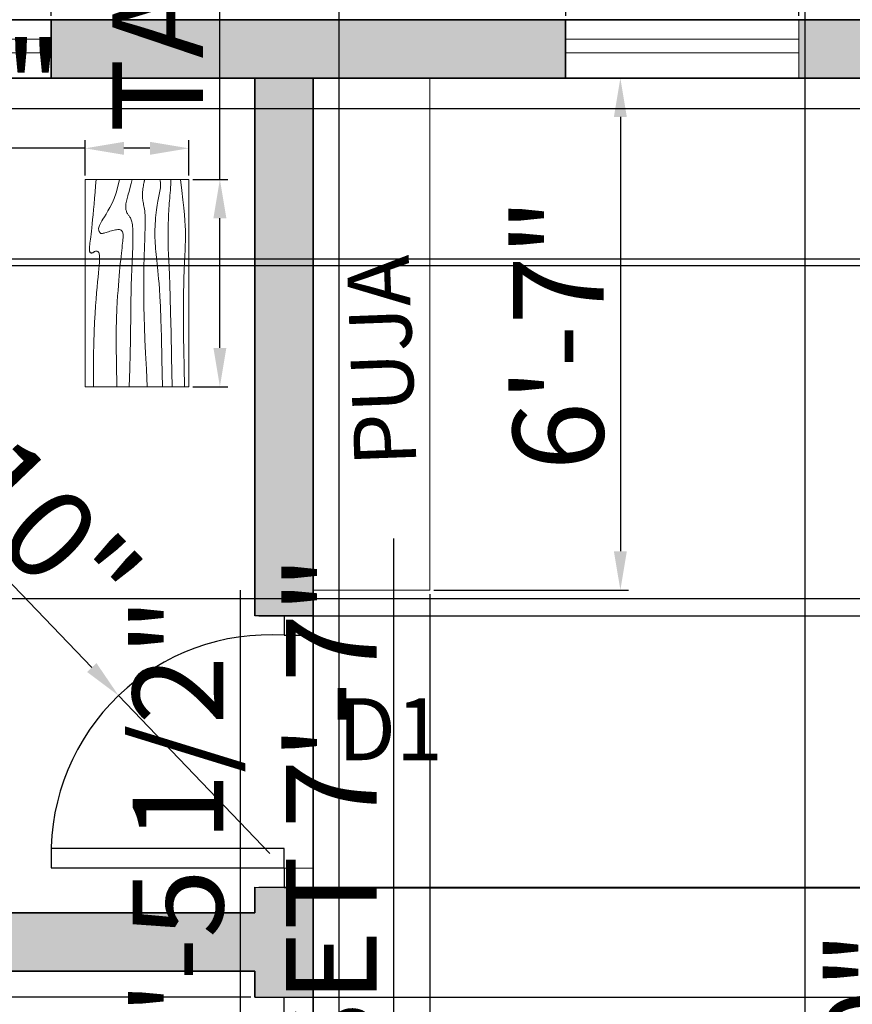
# Model space of a CAD drawing. Units: inches. Extents: x 2961 to 3748, y 1432 to 1961.
# Tile 6 of 9: x 3219 to 3348, y 1713 to 1865. Entities that reach past the tile are written whole.
import ezdxf
from ezdxf.enums import TextEntityAlignment as Align

# ---------------------------------------------------------------- set-up
doc = ezdxf.new("R2010")
doc.units = ezdxf.units.IN
for name, color, linetype, lineweight in [('A-ANNO-DIMS', 2, 'Continuous', 18), ('A-ANNO-TEXT', 7, 'Continuous', 18), ('A-AREA-IDEN', 7, 'Continuous', 18), ('A-DOOR', 3, 'Continuous', 25), ('A-FURN', 8, 'Continuous', 18), ('A-FURN-FIXD', 9, 'Continuous', 20), ('A-GLAZ', 4, 'Continuous', 18), ('A-WALL', 7, 'Continuous', 35), ('A-WALL-PATT', 252, 'Continuous', 13)]:
    doc.layers.add(name, color=color, linetype=linetype, lineweight=lineweight)
doc.styles.get("Standard").update_dxf_attribs({"font": 'arial.ttf'})
doc.dimstyles.new('ISO-25', dxfattribs={"dimtxt": 14, "dimasz": 6, "dimexe": 1.25, "dimexo": 0.625, "dimtad": 1, "dimlunit": 3, "dimtxsty": 'Standard', "dimcen": 2.5, "dimadec": 0, "dimazin": 0, "dimtfac": 1, "dimtmove": 0, "dimatfit": 3, "dimfxl": 1, "dimarcsym": 0})

# ---------------------------------------------------------------- blocks, each defined once
blk = doc.blocks.new('Table - Rectangular Woodgrain 60 x 30 in.')
for p, q in [((0, 0), (0, -30)), ((60, 0), (0, 0)), ((60, -30), (60, 0)), ((0, -30), (60, -30))]:
    blk.add_line(p, q)
for points in [[(0, -2.4), (4.8155, -2.418), (9.0302, -2.4688), (12.709, -2.5477), (15.9167, -2.65), (18.7181, -2.7711), (21.1781, -2.9063), (23.3616, -3.0508), (25.3333, -3.2), (27.1477, -3.3495), (28.8172, -3.4958), (30.3437, -3.636), (31.7291, -3.7667), (32.9756, -3.8849), (34.0849, -3.9875), (35.059, -4.0714), (35.9, -4.1334), (36.6114, -4.1711), (37.2041, -4.1854), (37.6906, -4.1779), (38.0833, -4.15), (38.3948, -4.1034), (38.6375, -4.0396), (38.8239, -3.9602), (38.9666, -3.8667), (39.0764, -3.7608), (39.1573, -3.6448), (39.2116, -3.521), (39.2416, -3.3917), (39.2498, -3.2593), (39.2385, -3.1261), (39.21, -2.9944), (39.1666, -2.8667), (39.111, -2.7447), (39.0468, -2.6281), (38.978, -2.5163), (38.9083, -2.4083), (38.8418, -2.3035), (38.7823, -2.201), (38.7337, -2.1001), (38.7, -2), (38.6844, -1.9003), (38.6875, -1.8021), (38.7094, -1.707), (38.75, -1.6167), (38.8094, -1.5326), (38.8875, -1.4563), (38.9844, -1.3893), (39.1, -1.3333), (39.2351, -1.2896), (39.3937, -1.2583), (39.5804, -1.2396), (39.8, -1.2333), (40.057, -1.2396), (40.3562, -1.2583), (40.7023, -1.2896), (41.1, -1.3333), (41.5547, -1.3895), (42.0755, -1.4573), (42.6721, -1.5361), (43.3542, -1.625), (44.1316, -1.7233), (45.014, -1.8302), (46.0114, -1.9449), (47.1333, -2.0667), (48.3862, -2.1947), (49.7625, -2.3281), (51.2513, -2.4663), (52.8416, -2.6083), (54.5226, -2.7535), (56.2833, -2.9011), (58.1127, -3.0501), (60, -3.2)], [(0, -9.2), (6.5759, -9.0858), (11.9385, -9.0365), (16.2527, -9.0418), (19.6833, -9.0917), (22.3952, -9.1759), (24.5531, -9.2844), (26.322, -9.4069), (27.8666, -9.5333), (29.3241, -9.6553), (30.7203, -9.7719), (32.0532, -9.8837), (33.3208, -9.9917), (34.5213, -10.0965), (35.6526, -10.199), (36.7128, -10.2999), (37.7, -10.4), (38.6129, -10.4996), (39.4531, -10.5969), (40.223, -10.6895), (40.925, -10.775), (41.5613, -10.8512), (42.1344, -10.9156), (42.6465, -10.966), (43.1, -11), (43.4976, -11.0158), (43.8437, -11.0136), (44.143, -10.9942), (44.4, -10.9583), (44.6195, -10.9069), (44.8062, -10.8406), (44.9648, -10.7603), (45.1, -10.6667), (45.2155, -10.5598), (45.3114, -10.4365), (45.3871, -10.2929), (45.4416, -10.125), (45.4743, -9.929), (45.4844, -9.7011), (45.4709, -9.4371), (45.4333, -9.1333), (45.3716, -8.7883), (45.2896, -8.4104), (45.1919, -8.0107), (45.0833, -7.6), (44.9685, -7.1893), (44.8521, -6.7896), (44.7388, -6.4117), (44.6333, -6.0667), (44.54, -5.7628), (44.4614, -5.4979), (44.4001, -5.2675), (44.3583, -5.0667), (44.3384, -4.8909), (44.3427, -4.7354), (44.3736, -4.5956), (44.4333, -4.4667), (44.5236, -4.3453), (44.6427, -4.2333), (44.7884, -4.1339), (44.9583, -4.05), (45.1501, -3.9849), (45.3614, -3.9417), (45.59, -3.9234), (45.8333, -3.9333), (46.0915, -3.9749), (46.3734, -4.0531), (46.6906, -4.1736), (47.0542, -4.3417), (47.4756, -4.5629), (47.9661, -4.8427), (48.5372, -5.1866), (49.2, -5.6), (49.9676, -6.0844), (50.8594, -6.625), (51.8965, -7.2031), (53.1, -7.8), (54.491, -8.3969), (56.0906, -8.975), (57.9199, -9.5156), (60, -10)], [(0, -12.8), (5.1847, -12.9322), (9.6213, -13.0323), (13.3963, -13.1059), (16.5958, -13.1583), (19.3063, -13.1952), (21.614, -13.2219), (23.6054, -13.2439), (25.3666, -13.2667), (26.9728, -13.2947), (28.4531, -13.3281), (29.8256, -13.3663), (31.1083, -13.4083), (32.3191, -13.4535), (33.476, -13.501), (34.597, -13.5501), (35.7, -13.6), (36.7984, -13.6497), (37.8875, -13.6979), (38.9578, -13.743), (40, -13.7833), (41.0047, -13.8174), (41.9625, -13.8438), (42.864, -13.8607), (43.7, -13.8667), (44.4631, -13.8604), (45.1552, -13.8417), (45.7801, -13.8104), (46.3416, -13.7667), (46.8439, -13.7104), (47.2906, -13.6417), (47.6858, -13.5604), (48.0333, -13.4667), (48.3375, -13.3608), (48.6042, -13.2448), (48.8396, -13.121), (49.05, -12.9917), (49.2417, -12.8593), (49.4208, -12.7261), (49.5937, -12.5944), (49.7667, -12.4667), (49.9452, -12.3451), (50.1323, -12.2313), (50.3303, -12.1268), (50.5416, -12.0333), (50.7686, -11.9524), (51.0135, -11.8854), (51.2788, -11.8341), (51.5666, -11.8), (51.8785, -11.7843), (52.2116, -11.7865), (52.562, -11.8059), (52.926, -11.8417), (53.2998, -11.8931), (53.6795, -11.9594), (54.0614, -12.0397), (54.4416, -12.1333), (54.8223, -12.2401), (55.2293, -12.3625), (55.6942, -12.5037), (56.2489, -12.6667), (56.9251, -12.8547), (57.7545, -13.0708), (58.7689, -13.3182), (60, -13.6)], [(0, -18), (5.124, -17.7273), (9.6609, -17.5057), (13.6705, -17.3303), (17.2125, -17.1958), (20.3467, -17.0973), (23.1328, -17.0297), (25.6307, -16.9878), (27.9, -16.9667), (29.9928, -16.9617), (31.9302, -16.9703), (33.7254, -16.9907), (35.3917, -17.0208), (36.9423, -17.0588), (38.3906, -17.1026), (39.7499, -17.1503), (41.0333, -17.2), (42.2519, -17.2496), (43.4073, -17.2969), (44.4986, -17.3395), (45.525, -17.375), (46.4858, -17.4012), (47.3802, -17.4156), (48.2074, -17.416), (48.9667, -17.4), (49.6583, -17.3662), (50.2872, -17.3167), (50.8595, -17.2547), (51.3812, -17.1833), (51.8584, -17.1057), (52.2971, -17.025), (52.7034, -16.9443), (53.0833, -16.8667), (53.443, -16.7951), (53.789, -16.7313), (54.128, -16.6768), (54.4666, -16.6334), (54.8115, -16.6024), (55.1693, -16.5854), (55.5465, -16.5841), (55.95, -16.6), (56.3828, -16.6337), (56.8346, -16.6823), (57.2915, -16.7418), (57.7396, -16.8084), (58.165, -16.878), (58.5539, -16.9469), (58.8924, -17.0111), (59.1666, -17.0667), (59.3679, -17.1107), (59.5078, -17.1438), (59.6032, -17.1675), (59.6708, -17.1833), (59.7275, -17.193), (59.7901, -17.1979), (59.8753, -17.1998), (60, -17.2)], [(0, -22.4), (8.0098, -22.2501), (14.4094, -22.1011), (19.4168, -21.9535), (23.25, -21.8083), (26.1269, -21.6663), (28.2656, -21.5281), (29.884, -21.3947), (31.2, -21.2667), (32.3967, -21.1448), (33.5172, -21.0292), (34.5697, -20.9198), (35.5625, -20.8167), (36.5037, -20.7198), (37.4015, -20.6292), (38.2642, -20.5448), (39.1, -20.4667), (39.9164, -20.3951), (40.7187, -20.3313), (41.5117, -20.2768), (42.3, -20.2333), (43.0883, -20.2024), (43.8812, -20.1854), (44.6836, -20.1841), (45.5, -20.2), (46.3328, -20.234), (47.1747, -20.2844), (48.0163, -20.3488), (48.8479, -20.425), (49.66, -20.5106), (50.4429, -20.6031), (51.1872, -20.7004), (51.8833, -20.8), (52.5246, -20.8999), (53.1166, -20.9995), (53.6681, -21.0983), (54.1875, -21.1958), (54.6834, -21.2919), (55.1646, -21.3859), (55.6394, -21.4777), (56.1167, -21.5667), (56.6028, -21.6515), (57.0961, -21.7266), (57.5929, -21.7852), (58.0896, -21.8208), (58.5823, -21.8268), (59.0674, -21.7964), (59.5412, -21.723), (60, -21.6)], [(0, -25.2), (8.6355, -25.0504), (15.7026, -24.9031), (21.4049, -24.7606), (25.9458, -24.625), (29.529, -24.4988), (32.3578, -24.3844), (34.6359, -24.284), (36.5667, -24.2), (38.3213, -24.1341), (39.9417, -24.0854), (41.437, -24.0523), (42.8167, -24.0333), (44.0901, -24.0268), (45.2667, -24.0313), (46.3557, -24.0451), (47.3667, -24.0667), (48.309, -24.0947), (49.1928, -24.1287), (50.0284, -24.168), (50.826, -24.2125), (51.5959, -24.2617), (52.3483, -24.3151), (53.0935, -24.3725), (53.8417, -24.4334), (54.6009, -24.497), (55.3699, -24.561), (56.1454, -24.6226), (56.9239, -24.6792), (57.7021, -24.7279), (58.4764, -24.7662), (59.2435, -24.7911), (60, -24.8)], [(0, -28.8), (5.6867, -28.6681), (10.45, -28.5698), (14.407, -28.5012), (17.675, -28.4584), (20.3711, -28.4374), (22.6125, -28.4344), (24.5164, -28.4455), (26.2, -28.4667), (27.762, -28.4947), (29.2276, -28.5281), (30.6033, -28.5663), (31.8958, -28.6084), (33.1118, -28.6535), (34.2578, -28.7011), (35.3405, -28.7501), (36.3666, -28.8), (37.3443, -28.8497), (38.288, -28.8974), (39.2137, -28.9412), (40.1375, -28.9792), (41.0753, -29.0093), (42.0432, -29.0297), (43.0572, -29.0384), (44.1333, -29.0333), (45.2936, -29.0114), (46.5843, -28.9641), (48.0579, -28.8816), (49.7666, -28.7542), (51.7629, -28.5721), (54.0989, -28.3255), (56.8272, -28.0048), (60, -27.6)]]:
    blk.add_lwpolyline(points)
blk = doc.blocks.new('*D14')
at = {"layer": 'A-ANNO-DIMS', "color": 0, "lineweight": -2, "transparency": 16777216}
for p, q in [((3054.27, 1865.26), (3054.27, 1895.31)), ((3603.27, 1865.26), (3603.27, 1895.31)), ((3060.27, 1894.06), (3597.27, 1894.06))]:
    blk.add_line(p, q, dxfattribs=at)
at = {"layer": 'A-ANNO-DIMS', "color": 0, "transparency": 16777216}
for points in [[(3060.27, 1895.06), (3060.27, 1893.06), (3054.27, 1894.06)], [(3597.27, 1895.06), (3597.27, 1893.06), (3603.27, 1894.06)]]:
    blk.add_solid(points, dxfattribs=at)
at = {"layer": 'Defpoints', "color": 0, "transparency": 16777216}
for p in [(3603.27, 1894.06), (3054.27, 1864.64), (3603.27, 1864.64)]:
    blk.add_point(p, dxfattribs=at)
at = {"layer": 'A-ANNO-DIMS', "color": 0, "transparency": 16777216, "insert": (3328.77, 1901.84), "char_height": 14, "attachment_point": 5}
blk.add_mtext('45\'-9"', dxfattribs=at)
blk = doc.blocks.new('WIN-36IN')
for p, q in [((0, 6), (36, 6)), ((0, 3.9), (36, 3.9))]:
    blk.add_line(p, q)
blk.add_lwpolyline([(36, 9), (0, 9), (0, 0), (36, 0)], close=True)
blk = doc.blocks.new('*D28')
at = {"layer": 'A-ANNO-DIMS', "color": 0, "lineweight": -2, "transparency": 16777216}
for p, q in [((3253.06, 1631.67), (3253.06, 1776.5)), ((3245.67, 1631.67), (3254.31, 1631.67)), ((3253.06, 1584.22), (3253.06, 1625.67)), ((3245.67, 1578.22), (3254.31, 1578.22))]:
    blk.add_line(p, q, dxfattribs=at)
at = {"layer": 'A-ANNO-DIMS', "color": 0, "transparency": 16777216}
for points in [[(3252.06, 1625.67), (3254.06, 1625.67), (3253.06, 1631.67)], [(3252.06, 1584.22), (3254.06, 1584.22), (3253.06, 1578.22)]]:
    blk.add_solid(points, dxfattribs=at)
at = {"layer": 'Defpoints', "color": 0, "transparency": 16777216}
for p in [(3245.04, 1631.67), (3253.06, 1631.67), (3245.04, 1578.22)]:
    blk.add_point(p, dxfattribs=at)
at = {"layer": 'A-ANNO-DIMS', "color": 0, "transparency": 16777216, "insert": (3245.19, 1707.08), "char_height": 14, "attachment_point": 5, "rotation": 90}
blk.add_mtext('TABLE 4\'-5 1/2"', dxfattribs=at)
blk = doc.blocks.new('*D30')
at = {"layer": 'A-ANNO-DIMS', "color": 0, "lineweight": -2, "transparency": 16777216}
for p, q in [((3249.85, 1839.99), (3249.85, 1952.2)), ((3245.67, 1839.99), (3251.1, 1839.99)), ((3249.85, 1813.95), (3249.85, 1833.99)), ((3245.67, 1807.95), (3251.1, 1807.95))]:
    blk.add_line(p, q, dxfattribs=at)
at = {"layer": 'A-ANNO-DIMS', "color": 0, "transparency": 16777216}
for points in [[(3248.85, 1833.99), (3250.85, 1833.99), (3249.85, 1839.99)], [(3248.85, 1813.95), (3250.85, 1813.95), (3249.85, 1807.95)]]:
    blk.add_solid(points, dxfattribs=at)
at = {"layer": 'Defpoints', "color": 0, "transparency": 16777216}
for p in [(3245.04, 1839.99), (3249.85, 1839.99), (3245.04, 1807.95)]:
    blk.add_point(p, dxfattribs=at)
at = {"layer": 'A-ANNO-DIMS', "color": 0, "transparency": 16777216, "insert": (3242.07, 1899.09), "char_height": 14, "attachment_point": 5, "rotation": 90}
blk.add_mtext('TABLE 2\'-8"', dxfattribs=at)
blk = doc.blocks.new('*D31')
at = {"layer": 'A-ANNO-DIMS', "color": 0, "lineweight": -2, "transparency": 16777216}
for p, q in [((3229.02, 1840.61), (3229.02, 1846.04)), ((3245.04, 1840.61), (3245.04, 1846.04)), ((3229.02, 1844.79), (3185.88, 1844.79)), ((3239.04, 1844.79), (3235.02, 1844.79))]:
    blk.add_line(p, q, dxfattribs=at)
at = {"layer": 'A-ANNO-DIMS', "color": 0, "transparency": 16777216}
for points in [[(3235.02, 1845.79), (3235.02, 1843.79), (3229.02, 1844.79)], [(3239.04, 1845.79), (3239.04, 1843.79), (3245.04, 1844.79)]]:
    blk.add_solid(points, dxfattribs=at)
at = {"layer": 'Defpoints', "color": 0, "transparency": 16777216}
for p in [(3229.02, 1844.79), (3229.02, 1839.99), (3245.04, 1839.99)]:
    blk.add_point(p, dxfattribs=at)
at = {"layer": 'A-ANNO-DIMS', "color": 0, "transparency": 16777216, "insert": (3204.45, 1852.45), "char_height": 14, "attachment_point": 5}
blk.add_mtext('1\'-4"', dxfattribs=at)
blk = doc.blocks.new('*D44')
at = {"layer": 'A-ANNO-DIMS', "color": 0, "lineweight": -2, "transparency": 16777216}
for p, q in [((3276.73, 1623.38), (3276.73, 1784.51)), ((3289.75, 1623.38), (3275.48, 1623.38)), ((3276.73, 1538.38), (3276.73, 1617.38)), ((3289.75, 1532.38), (3275.48, 1532.38))]:
    blk.add_line(p, q, dxfattribs=at)
at = {"layer": 'A-ANNO-DIMS', "color": 0, "transparency": 16777216}
for points in [[(3275.73, 1617.38), (3277.73, 1617.38), (3276.73, 1623.38)], [(3275.73, 1538.38), (3277.73, 1538.38), (3276.73, 1532.38)]]:
    blk.add_solid(points, dxfattribs=at)
at = {"layer": 'Defpoints', "color": 0, "transparency": 16777216}
for p in [(3276.73, 1623.38), (3290.38, 1623.38), (3290.38, 1532.38)]:
    blk.add_point(p, dxfattribs=at)
at = {"layer": 'A-ANNO-DIMS', "color": 0, "transparency": 16777216, "insert": (3268.87, 1706.94), "char_height": 14, "attachment_point": 5, "rotation": 90}
blk.add_mtext('DINING SET 7\'-7"', dxfattribs=at)
blk = doc.blocks.new('*D50')
at = {"layer": 'A-ANNO-DIMS', "color": 0, "lineweight": -2, "transparency": 16777216}
for p, q in [((3282.89, 1855.64), (3312.97, 1855.64)), ((3311.72, 1849.64), (3311.72, 1782.53)), ((3282.89, 1776.53), (3312.97, 1776.53))]:
    blk.add_line(p, q, dxfattribs=at)
at = {"layer": 'A-ANNO-DIMS', "color": 0, "transparency": 16777216}
for points in [[(3310.72, 1849.64), (3312.72, 1849.64), (3311.72, 1855.64)], [(3310.72, 1782.53), (3312.72, 1782.53), (3311.72, 1776.53)]]:
    blk.add_solid(points, dxfattribs=at)
at = {"layer": 'Defpoints', "color": 0, "transparency": 16777216}
for p in [(3282.27, 1855.64), (3282.27, 1776.53), (3311.72, 1776.53)]:
    blk.add_point(p, dxfattribs=at)
at = {"layer": 'A-ANNO-DIMS', "color": 0, "transparency": 16777216, "insert": (3303.94, 1816.09), "char_height": 14, "attachment_point": 5, "rotation": 90}
blk.add_mtext('6\'-7"', dxfattribs=at)
blk = doc.blocks.new('*D52')
at = {"layer": 'A-ANNO-DIMS', "color": 0, "lineweight": -2, "transparency": 16777216}
for p, q in [((3360.27, 1678.21), (3360.27, 1721.36)), ((3389.1, 1672.21), (3359.02, 1672.21)), ((3360.27, 1660.05), (3360.27, 1672.21)), ((3389.1, 1660.05), (3359.02, 1660.05)), ((3360.27, 1654.05), (3360.27, 1648.05))]:
    blk.add_line(p, q, dxfattribs=at)
at = {"layer": 'A-ANNO-DIMS', "color": 0, "transparency": 16777216}
for points in [[(3359.27, 1678.21), (3361.27, 1678.21), (3360.27, 1672.21)], [(3359.27, 1654.05), (3361.27, 1654.05), (3360.27, 1660.05)]]:
    blk.add_solid(points, dxfattribs=at)
at = {"layer": 'Defpoints', "color": 0, "transparency": 16777216}
for p in [(3360.27, 1672.21), (3389.72, 1672.21), (3389.72, 1660.05)]:
    blk.add_point(p, dxfattribs=at)
at = {"layer": 'A-ANNO-DIMS', "color": 0, "transparency": 16777216, "insert": (3352.5, 1702.78), "char_height": 14, "attachment_point": 5, "rotation": 90}
blk.add_mtext('1\'-0"', dxfattribs=at)
blk = doc.blocks.new('*D53')
at = {"layer": 'A-ANNO-DIMS', "color": 0, "lineweight": -2, "transparency": 16777216}
for p, q in [((3123.27, 1855.01), (3123.27, 1473.94)), ((3187.8, 1855.01), (3187.8, 1473.94)), ((3129.27, 1475.19), (3181.8, 1475.19)), ((3187.8, 1475.19), (3264.89, 1475.19))]:
    blk.add_line(p, q, dxfattribs=at)
at = {"layer": 'A-ANNO-DIMS', "color": 0, "transparency": 16777216}
for points in [[(3129.27, 1476.19), (3129.27, 1474.19), (3123.27, 1475.19)], [(3181.8, 1476.19), (3181.8, 1474.19), (3187.8, 1475.19)]]:
    blk.add_solid(points, dxfattribs=at)
at = {"layer": 'Defpoints', "color": 0, "transparency": 16777216}
for p in [(3123.27, 1855.64), (3187.8, 1855.64), (3187.8, 1475.19)]:
    blk.add_point(p, dxfattribs=at)
at = {"layer": 'A-ANNO-DIMS', "color": 0, "transparency": 16777216, "insert": (3229.35, 1483.05), "char_height": 14, "attachment_point": 5}
blk.add_mtext('5\'-4 1/2"', dxfattribs=at)
blk = doc.blocks.new('*D54')
at = {"layer": 'A-ANNO-DIMS', "color": 0, "lineweight": -2, "transparency": 16777216}
for p, q in [((3223.8, 1865.26), (3223.8, 1933.63)), ((3229.8, 1932.38), (3297.27, 1932.38)), ((3303.27, 1865.26), (3303.27, 1933.63))]:
    blk.add_line(p, q, dxfattribs=at)
at = {"layer": 'A-ANNO-DIMS', "color": 0, "transparency": 16777216}
for points in [[(3229.8, 1933.38), (3229.8, 1931.38), (3223.8, 1932.38)], [(3297.27, 1933.38), (3297.27, 1931.38), (3303.27, 1932.38)]]:
    blk.add_solid(points, dxfattribs=at)
at = {"layer": 'Defpoints', "color": 0, "transparency": 16777216}
for p in [(3303.27, 1932.38), (3223.8, 1864.64), (3303.27, 1864.64)]:
    blk.add_point(p, dxfattribs=at)
at = {"layer": 'A-ANNO-DIMS', "color": 0, "transparency": 16777216, "insert": (3263.53, 1940.24), "char_height": 14, "attachment_point": 5}
blk.add_mtext('6\'-7 1/2"', dxfattribs=at)
blk = doc.blocks.new('*D55')
at = {"layer": 'A-ANNO-DIMS', "color": 0, "lineweight": -2, "transparency": 16777216}
for p, q in [((3339.27, 1865.26), (3339.27, 1933.63)), ((3345.27, 1932.38), (3429.27, 1932.38)), ((3435.27, 1865.26), (3435.27, 1933.63))]:
    blk.add_line(p, q, dxfattribs=at)
at = {"layer": 'A-ANNO-DIMS', "color": 0, "transparency": 16777216}
for points in [[(3345.27, 1933.38), (3345.27, 1931.38), (3339.27, 1932.38)], [(3429.27, 1933.38), (3429.27, 1931.38), (3435.27, 1932.38)]]:
    blk.add_solid(points, dxfattribs=at)
at = {"layer": 'Defpoints', "color": 0, "transparency": 16777216}
for p in [(3435.27, 1932.38), (3339.27, 1864.64), (3435.27, 1864.64)]:
    blk.add_point(p, dxfattribs=at)
at = {"layer": 'A-ANNO-DIMS', "color": 0, "transparency": 16777216, "insert": (3387.27, 1940.15), "char_height": 14, "attachment_point": 5}
blk.add_mtext('8\'-0"', dxfattribs=at)
blk = doc.blocks.new('*D64')
at = {"layer": 'A-ANNO-DIMS', "color": 0, "lineweight": -2, "transparency": 16777216}
for p, q in [((3509.64, 1855.64), (3023.57, 1855.64)), ((3024.82, 1849.64), (3024.82, 1833.64)), ((3509.64, 1827.64), (3023.57, 1827.64)), ((3024.82, 1827.64), (3024.82, 1782.93))]:
    blk.add_line(p, q, dxfattribs=at)
at = {"layer": 'A-ANNO-DIMS', "color": 0, "transparency": 16777216}
for points in [[(3023.82, 1849.64), (3025.82, 1849.64), (3024.82, 1855.64)], [(3023.82, 1833.64), (3025.82, 1833.64), (3024.82, 1827.64)]]:
    blk.add_solid(points, dxfattribs=at)
at = {"layer": 'Defpoints', "color": 0, "transparency": 16777216}
for p in [(3510.27, 1855.64), (3024.82, 1827.64), (3510.27, 1827.64)]:
    blk.add_point(p, dxfattribs=at)
at = {"layer": 'A-ANNO-DIMS', "color": 0, "transparency": 16777216, "insert": (3017.16, 1802.29), "char_height": 14, "attachment_point": 5, "rotation": 90}
blk.add_mtext('2\'-4"', dxfattribs=at)
blk = doc.blocks.new('*D69')
at = {"layer": 'A-ANNO-DIMS', "color": 0, "lineweight": -2, "transparency": 16777216}
for p, q in [((3268.27, 1646.26), (3268.27, 1933.63)), ((3274.27, 1932.38), (3334.27, 1932.38)), ((3340.27, 1646.26), (3340.27, 1933.63))]:
    blk.add_line(p, q, dxfattribs=at)
at = {"layer": 'A-ANNO-DIMS', "color": 0, "transparency": 16777216}
for points in [[(3274.27, 1933.38), (3274.27, 1931.38), (3268.27, 1932.38)], [(3334.27, 1933.38), (3334.27, 1931.38), (3340.27, 1932.38)]]:
    blk.add_solid(points, dxfattribs=at)
at = {"layer": 'Defpoints', "color": 0, "transparency": 16777216}
for p in [(3340.27, 1932.38), (3268.27, 1645.64), (3340.27, 1645.64)]:
    blk.add_point(p, dxfattribs=at)
at = {"layer": 'A-ANNO-DIMS', "color": 0, "transparency": 16777216, "insert": (3304.27, 1940.15), "char_height": 14, "attachment_point": 5}
blk.add_mtext('6\'-0"', dxfattribs=at)
blk = doc.blocks.new('*D71')
at = {"layer": 'A-ANNO-DIMS', "color": 0, "lineweight": -2, "transparency": 16777216}
for p, q in [((3255.89, 1772.53), (3633.97, 1772.53)), ((3632.72, 1736.64), (3632.72, 1766.53)), ((3255.89, 1730.64), (3633.97, 1730.64))]:
    blk.add_line(p, q, dxfattribs=at)
at = {"layer": 'A-ANNO-DIMS', "color": 0, "transparency": 16777216}
for points in [[(3631.72, 1766.53), (3633.72, 1766.53), (3632.72, 1772.53)], [(3631.72, 1736.64), (3633.72, 1736.64), (3632.72, 1730.64)]]:
    blk.add_solid(points, dxfattribs=at)
at = {"layer": 'Defpoints', "color": 0, "transparency": 16777216}
for p in [(3255.27, 1772.53), (3632.72, 1772.53), (3255.27, 1730.64)]:
    blk.add_point(p, dxfattribs=at)
at = {"layer": 'A-ANNO-DIMS', "color": 0, "transparency": 16777216, "insert": (3624.94, 1751.59), "char_height": 14, "attachment_point": 5, "rotation": 90}
blk.add_mtext('3\'-6"', dxfattribs=at)
blk = doc.blocks.new('*D72')
at = {"layer": 'A-ANNO-DIMS', "color": 0, "lineweight": -2, "transparency": 16777216}
for p, q in [((3255.89, 1713.64), (3633.97, 1713.64)), ((3632.72, 1677.64), (3632.72, 1707.64)), ((3255.89, 1671.64), (3633.97, 1671.64))]:
    blk.add_line(p, q, dxfattribs=at)
at = {"layer": 'A-ANNO-DIMS', "color": 0, "transparency": 16777216}
for points in [[(3631.72, 1707.64), (3633.72, 1707.64), (3632.72, 1713.64)], [(3631.72, 1677.64), (3633.72, 1677.64), (3632.72, 1671.64)]]:
    blk.add_solid(points, dxfattribs=at)
at = {"layer": 'Defpoints', "color": 0, "transparency": 16777216}
for p in [(3255.27, 1713.64), (3632.72, 1713.64), (3255.27, 1671.64)]:
    blk.add_point(p, dxfattribs=at)
at = {"layer": 'A-ANNO-DIMS', "color": 0, "transparency": 16777216, "insert": (3624.94, 1692.64), "char_height": 14, "attachment_point": 5, "rotation": 90}
blk.add_mtext('3\'-6"', dxfattribs=at)
blk = doc.blocks.new('*D75')
at = {"layer": 'A-ANNO-DIMS', "color": 0, "lineweight": -2, "transparency": 16777216}
for p, q in [((3024.82, 1723.64), (3024.82, 1729.64)), ((3254.64, 1717.64), (3023.57, 1717.64)), ((3024.82, 1717.64), (3024.82, 1713.64)), ((3254.64, 1713.64), (3023.57, 1713.64)), ((3024.82, 1707.64), (3024.82, 1663.17))]:
    blk.add_line(p, q, dxfattribs=at)
at = {"layer": 'A-ANNO-DIMS', "color": 0, "transparency": 16777216}
for points in [[(3023.82, 1723.64), (3025.82, 1723.64), (3024.82, 1717.64)], [(3023.82, 1707.64), (3025.82, 1707.64), (3024.82, 1713.64)]]:
    blk.add_solid(points, dxfattribs=at)
at = {"layer": 'Defpoints', "color": 0, "transparency": 16777216}
for p in [(3255.27, 1717.64), (3024.82, 1713.64), (3255.27, 1713.64)]:
    blk.add_point(p, dxfattribs=at)
at = {"layer": 'A-ANNO-DIMS', "color": 0, "transparency": 16777216, "insert": (3017.04, 1682.41), "char_height": 14, "attachment_point": 5, "rotation": 90}
blk.add_mtext('0\'-4"', dxfattribs=at)
blk = doc.blocks.new('*D76')
at = {"layer": 'A-ANNO-DIMS', "color": 0, "lineweight": -2, "transparency": 16777216}
for p, q in [((3632.72, 1730.53), (3632.72, 1773.68)), ((3264.89, 1730.53), (3633.97, 1730.53)), ((3632.72, 1719.64), (3632.72, 1724.53)), ((3264.89, 1713.64), (3633.97, 1713.64))]:
    blk.add_line(p, q, dxfattribs=at)
at = {"layer": 'A-ANNO-DIMS', "color": 0, "transparency": 16777216}
for points in [[(3631.72, 1724.53), (3633.72, 1724.53), (3632.72, 1730.53)], [(3631.72, 1719.64), (3633.72, 1719.64), (3632.72, 1713.64)]]:
    blk.add_solid(points, dxfattribs=at)
at = {"layer": 'Defpoints', "color": 0, "transparency": 16777216}
for p in [(3264.27, 1730.53), (3632.72, 1730.53), (3264.27, 1713.64)]:
    blk.add_point(p, dxfattribs=at)
at = {"layer": 'A-ANNO-DIMS', "color": 0, "transparency": 16777216, "insert": (3624.94, 1755.11), "char_height": 14, "attachment_point": 5, "rotation": 90}
blk.add_mtext('1\'-5"', dxfattribs=at)
blk = doc.blocks.new('*D77')
at = {"layer": 'A-ANNO-DIMS', "color": 0, "lineweight": -2, "transparency": 16777216}
for p, q in [((3264.27, 1775.91), (3264.27, 1473.94)), ((3282.27, 1775.91), (3282.27, 1473.94)), ((3270.27, 1475.19), (3276.27, 1475.19)), ((3282.27, 1475.19), (3325.41, 1475.19))]:
    blk.add_line(p, q, dxfattribs=at)
at = {"layer": 'A-ANNO-DIMS', "color": 0, "transparency": 16777216}
for points in [[(3270.27, 1476.19), (3270.27, 1474.19), (3264.27, 1475.19)], [(3276.27, 1476.19), (3276.27, 1474.19), (3282.27, 1475.19)]]:
    blk.add_solid(points, dxfattribs=at)
at = {"layer": 'Defpoints', "color": 0, "transparency": 16777216}
for p in [(3264.27, 1776.53), (3282.27, 1776.53), (3282.27, 1475.19)]:
    blk.add_point(p, dxfattribs=at)
at = {"layer": 'A-ANNO-DIMS', "color": 0, "transparency": 16777216, "insert": (3306.84, 1482.96), "char_height": 14, "attachment_point": 5}
blk.add_mtext('1\'-6"', dxfattribs=at)
blk = doc.blocks.new('*D83')
at = {"layer": 'A-ANNO-DIMS', "color": 0, "lineweight": -2, "transparency": 16777216}
for p, q in [((3123.89, 1855.64), (3633.97, 1855.64)), ((3632.72, 1781.22), (3632.72, 1849.64)), ((3123.89, 1775.22), (3633.97, 1775.22))]:
    blk.add_line(p, q, dxfattribs=at)
at = {"layer": 'A-ANNO-DIMS', "color": 0, "transparency": 16777216}
for points in [[(3631.72, 1849.64), (3633.72, 1849.64), (3632.72, 1855.64)], [(3631.72, 1781.22), (3633.72, 1781.22), (3632.72, 1775.22)]]:
    blk.add_solid(points, dxfattribs=at)
at = {"layer": 'Defpoints', "color": 0, "transparency": 16777216}
for p in [(3123.27, 1855.64), (3632.72, 1855.64), (3123.27, 1775.22)]:
    blk.add_point(p, dxfattribs=at)
at = {"layer": 'A-ANNO-DIMS', "color": 0, "transparency": 16777216, "insert": (3624.85, 1815.43), "char_height": 14, "attachment_point": 5, "rotation": 90}
blk.add_mtext('6\'-8 1/2"', dxfattribs=at)
blk = doc.blocks.new('*D86')
at = {"layer": 'A-ANNO-DIMS', "color": 0, "lineweight": -2, "transparency": 16777216}
for p, q in [((3091.52, 1850.93), (3633.97, 1850.93)), ((3632.72, 1844.93), (3632.72, 1832.66)), ((3082.42, 1826.66), (3633.97, 1826.66)), ((3632.72, 1826.66), (3632.72, 1749.34))]:
    blk.add_line(p, q, dxfattribs=at)
at = {"layer": 'A-ANNO-DIMS', "color": 0, "transparency": 16777216}
for points in [[(3631.72, 1844.93), (3633.72, 1844.93), (3632.72, 1850.93)], [(3631.72, 1832.66), (3633.72, 1832.66), (3632.72, 1826.66)]]:
    blk.add_solid(points, dxfattribs=at)
at = {"layer": 'Defpoints', "color": 0, "transparency": 16777216}
for p in [(3090.9, 1850.93), (3081.8, 1826.66), (3632.72, 1826.66)]:
    blk.add_point(p, dxfattribs=at)
at = {"layer": 'A-ANNO-DIMS', "color": 0, "transparency": 16777216, "insert": (3624.85, 1785), "char_height": 14, "attachment_point": 5, "rotation": 90}
blk.add_mtext('2\'-0 1/2"', dxfattribs=at)
blk = doc.blocks.new('*D94')
at = {"layer": 'A-ANNO-DIMS', "color": 0, "lineweight": -2, "transparency": 16777216}
for p, q in [((3182.5, 1814.2), (3230.05, 1764.56)), ((3257.56, 1735.84), (3234.2, 1760.22))]:
    blk.add_line(p, q, dxfattribs=at)
at = {"layer": 'A-ANNO-DIMS', "color": 0, "transparency": 16777216}
blk.add_solid([(3230.78, 1765.25), (3229.33, 1763.87), (3234.2, 1760.22)], dxfattribs=at)
at = {"layer": 'Defpoints', "color": 0, "transparency": 16777216}
for p in [(3234.2, 1760.22), (3257.56, 1735.84)]:
    blk.add_point(p, dxfattribs=at)
at = {"layer": 'A-ANNO-DIMS', "color": 0, "transparency": 16777216, "insert": (3209.82, 1796.92), "char_height": 14, "attachment_point": 5, "rotation": 313.7658}
blk.add_mtext('R2\'-10"', dxfattribs=at)

msp = doc.modelspace()

# ---------------------------------------------------------------- hatches: boundary and pattern name
at = {"layer": 'A-WALL-PATT'}
h = msp.add_hatch(color=256, dxfattribs=at)
h.set_gradient(color1=(41, 49, 137), color2=(41, 49, 137), tint=1)
h.paths.add_polyline_path([(3255.267, 1671.639), (3255.267, 1513.639), (3251.267, 1513.639), (3251.267, 1504.639), (3268.267, 1504.639), (3268.267, 1513.639), (3264.267, 1513.639), (3264.267, 1671.639), (3259.767, 1671.639)])
h.paths.add_polyline_path([(3063.267, 1513.639), (3063.267, 1677.639), (3054.267, 1677.639), (3054.267, 1504.639), (3215.267, 1504.639), (3215.267, 1513.639)])
h.paths.add_polyline_path([(3304.267, 1513.639), (3304.267, 1504.639), (3456.267, 1504.639), (3456.267, 1513.639), (3390.267, 1513.639), (3390.267, 1605.639), (3384.267, 1605.639), (3384.267, 1513.639)])
h.paths.add_polyline_path([(3510.267, 1605.639), (3510.267, 1513.639), (3492.267, 1513.639), (3492.267, 1504.639), (3546.267, 1504.639), (3546.267, 1513.639), (3519.267, 1513.639), (3519.267, 1605.639)])
h.paths.add_polyline_path([(3340.267, 1654.639), (3340.267, 1645.639), (3510.267, 1645.639), (3510.267, 1641.639), (3519.267, 1641.639), (3519.267, 1658.639), (3510.267, 1658.639), (3510.267, 1654.639)])
h.paths.add_polyline_path([(3223.801, 1864.639), (3223.801, 1855.639), (3255.267, 1855.639), (3255.267, 1772.534), (3264.267, 1772.534), (3264.267, 1855.639), (3303.267, 1855.639), (3303.267, 1864.639)])
h.paths.add_polyline_path([(3339.267, 1864.639), (3339.267, 1855.639), (3435.267, 1855.639), (3435.267, 1864.639)])
h.paths.add_polyline_path([(3471.267, 1864.639), (3471.267, 1855.639), (3510.267, 1855.639), (3510.267, 1827.639), (3519.267, 1827.639), (3519.267, 1864.639)])
h.paths.add_polyline_path([(3510.267, 1767.639), (3510.267, 1739.639), (3519.267, 1739.639), (3519.267, 1767.639)])
h.paths.add_polyline_path([(3123.267, 1726.639), (3123.267, 1855.639), (3187.801, 1855.639), (3187.801, 1864.639), (3054.267, 1864.639), (3054.267, 1837.201), (3063.267, 1837.201), (3063.267, 1855.639), (3117.267, 1855.639), (3117.267, 1726.639), (3103.267, 1726.639), (3103.267, 1717.639), (3255.267, 1717.639), (3255.267, 1713.639), (3264.267, 1713.639), (3264.267, 1730.534), (3255.267, 1730.639), (3255.267, 1726.639)])
h.paths.add_polyline_path([(3597.267, 1654.639), (3597.267, 1513.639), (3570.267, 1513.639), (3570.267, 1504.639), (3603.267, 1504.639), (3603.267, 1654.639)])
h.paths.add_polyline_path([(3054.267, 1813.201), (3054.267, 1713.639), (3063.267, 1713.639), (3063.267, 1717.639), (3069.267, 1717.639), (3069.267, 1726.639), (3063.267, 1726.639), (3063.267, 1813.201)], flags=17)

# ---------------------------------------------------------------- linework, layer by layer
at = {"layer": 'A-DOOR'}
for p, q in [((3264.267, 1772.534), (3255.267, 1772.534)), ((3259.767, 1772.534), (3259.767, 1769.534)), ((3259.767, 1769.534), (3264.267, 1769.534)), ((3259.801, 1733.586), (3259.766, 1730.586)), ((3259.801, 1733.586), (3264.301, 1733.534)), ((3255.267, 1730.639), (3264.266, 1730.534)), ((3255.267, 1713.639), (3264.267, 1713.639)), ((3259.767, 1710.639), (3259.767, 1713.639))]:
    msp.add_line(p, q, dxfattribs=at)
msp.add_lwpolyline([(3259.801, 1733.586), (3259.801, 1736.586), (3223.801, 1736.586), (3223.801, 1733.586)], close=True, dxfattribs=at)
msp.add_arc((3257.563, 1735.836), 33.77, 86.2585, 181.27259, dxfattribs=at)
at = {"layer": 'A-FURN-FIXD'}
for p, q in [((3282.267, 1776.534), (3282.267, 1855.639)), ((3264.267, 1776.534), (3282.267, 1776.534))]:
    msp.add_line(p, q, dxfattribs=at)
at = {"layer": 'A-WALL'}
for p, q in [((3054.267, 1864.639), (3519.267, 1864.639)), ((3223.801, 1864.639), (3223.801, 1855.639)), ((3303.267, 1855.639), (3303.267, 1864.639)), ((3255.267, 1855.639), (3123.267, 1855.639)), ((3255.267, 1772.534), (3255.267, 1855.639)), ((3264.267, 1513.639), (3264.267, 1855.639)), ((3510.267, 1855.639), (3264.267, 1855.639)), ((3264.267, 1772.534), (3264.267, 1776.534)), ((3255.267, 1726.639), (3255.267, 1730.639)), ((3255.267, 1726.639), (3123.267, 1726.639)), ((3255.267, 1717.639), (3063.267, 1717.639)), ((3255.267, 1713.639), (3255.267, 1717.639))]:
    msp.add_line(p, q, dxfattribs=at)

# ---------------------------------------------------------------- block references
at = {"layer": 'A-FURN', "xscale": 0.5339225242797914, "yscale": 0.5339225242797914, "zscale": 0.5339225242797914, "rotation": 90}
msp.add_blockref('Table - Rectangular Woodgrain 60 x 30 in.', (3229.024, 1807.952), dxfattribs=at)
at = {"layer": 'A-GLAZ'}
for p in [(3187.801, 1855.639), (3303.267, 1855.639)]:
    msp.add_blockref('WIN-36IN', p, dxfattribs=at)

# ---------------------------------------------------------------- texts
at = {"layer": 'A-ANNO-TEXT'}
msp.add_text('D1', height=9.5707, dxfattribs=at).set_placement((3268.074, 1750.24))
at = {"layer": 'A-AREA-IDEN'}
msp.add_text('PUJA', height=9.5707, rotation=92.15165, dxfattribs=at).set_placement((3279.617, 1812.097), align=Align.CENTER)

# ---------------------------------------------------------------- dimensions: what is measured, and where the dimension line sits
at = {"layer": 'A-ANNO-DIMS'}
for base, p1, p2, override, picture, middle in [((3303.267, 1932.38), (3223.801, 1864.639), (3303.267, 1864.639), {"dimdec": 1, "dimlfac": 1, "dimrnd": 0, "dimzin": 1, "dimdsep": 46, "dimlunit": 4, "dimfrac": 2}, '*D54', (3263.534, 1940.244)), ((3340.267, 1932.38), (3268.267, 1645.639), (3340.267, 1645.639), {"dimdec": 1, "dimlfac": 1, "dimrnd": 0, "dimzin": 1, "dimdsep": 46, "dimlunit": 4, "dimfrac": 2}, '*D69', (3304.267, 1940.153)), ((3435.267, 1932.38), (3339.267, 1864.639), (3435.267, 1864.639), {"dimdec": 1, "dimlfac": 1, "dimrnd": 0, "dimzin": 1, "dimdsep": 46, "dimlunit": 4, "dimfrac": 2}, '*D55', (3387.267, 1940.153)), ((3603.267, 1894.063), (3054.267, 1864.639), (3603.267, 1864.639), {"dimclrd": 0, "dimclre": 0, "dimclrt": 0}, '*D14', (3328.767, 1901.836)), ((3187.801, 1475.189), (3123.267, 1855.639), (3187.801, 1855.639), {"dimdec": 1, "dimlfac": 1, "dimrnd": 0, "dimzin": 1, "dimdsep": 46, "dimlunit": 4, "dimfrac": 2}, '*D53', (3229.345, 1483.052)), ((3282.267, 1475.189), (3264.267, 1776.534), (3282.267, 1776.534), {"dimdec": 1, "dimlfac": 1, "dimrnd": 0, "dimzin": 1, "dimdsep": 46, "dimlunit": 4, "dimfrac": 2}, '*D77', (3306.841, 1482.962))]:
    dim = msp.add_linear_dim(base=base, p1=p1, p2=p2, dimstyle='ISO-25', override=override, dxfattribs=at)
    dim.commit()
    dim.dimension.update_dxf_attribs({"geometry": picture, "text_midpoint": middle})
for base, p1, p2, text, picture, middle in [((3249.847, 1839.987), (3245.042, 1807.952), (3245.042, 1839.987), 'TABLE <>', '*D30', (3242.074, 1899.093)), ((3276.73, 1623.382), (3290.38, 1532.382), (3290.38, 1623.382), 'DINING SET <>', '*D44', (3268.866, 1706.945)), ((3253.058, 1631.667), (3245.042, 1578.224), (3245.042, 1631.667), 'TABLE <>', '*D28', (3245.195, 1707.084))]:
    dim = msp.add_linear_dim(base=base, p1=p1, p2=p2, angle=90, text=text, dimstyle='ISO-25', override={"dimdec": 1, "dimlfac": 1, "dimrnd": 0, "dimzin": 1, "dimdsep": 46, "dimlunit": 4, "dimfrac": 2}, dxfattribs=at)
    dim.commit()
    dim.dimension.update_dxf_attribs({"geometry": picture, "text_midpoint": middle})
for base, p1, p2, angle, picture, middle in [((3229.024, 1844.793), (3245.042, 1839.987), (3229.024, 1839.987), 180, '*D31', (3204.45, 1852.446)), ((3024.817, 1827.639), (3510.267, 1855.639), (3510.267, 1827.639), 90, '*D64', (3017.163, 1802.287)), ((3632.717, 1855.639), (3123.267, 1775.22), (3123.267, 1855.639), 90, '*D83', (3624.853, 1815.429)), ((3311.717, 1776.534), (3282.267, 1855.639), (3282.267, 1776.534), 270, '*D50', (3303.944, 1816.087)), ((3632.717, 1826.664), (3090.897, 1850.93), (3081.797, 1826.664), 90, '*D86', (3624.853, 1785)), ((3632.717, 1730.534), (3264.267, 1713.639), (3264.266, 1730.534), 90, '*D76', (3624.944, 1755.108)), ((3632.717, 1772.534), (3255.267, 1730.639), (3255.267, 1772.534), 90, '*D71', (3624.939, 1751.587)), ((3024.817, 1713.639), (3255.267, 1717.639), (3255.267, 1713.639), 90, '*D75', (3017.044, 1682.406)), ((3360.274, 1672.208), (3389.724, 1660.049), (3389.724, 1672.208), 90, '*D52', (3352.501, 1702.782)), ((3632.717, 1713.639), (3255.267, 1671.639), (3255.267, 1713.639), 90, '*D72', (3624.939, 1692.639))]:
    dim = msp.add_linear_dim(base=base, p1=p1, p2=p2, angle=angle, dimstyle='ISO-25', override={"dimdec": 1, "dimlfac": 1, "dimrnd": 0, "dimzin": 1, "dimdsep": 46, "dimlunit": 4, "dimfrac": 2}, dxfattribs=at)
    dim.commit()
    dim.dimension.update_dxf_attribs({"geometry": picture, "text_midpoint": middle})
dim = msp.add_radius_dim(center=(3257.563, 1735.836), mpoint=(3234.204, 1760.224), dimstyle='ISO-25', override={"dimdec": 1, "dimlfac": 1, "dimrnd": 0, "dimzin": 1, "dimdsep": 46, "dimlunit": 4, "dimfrac": 2}, dxfattribs=at)
dim.commit()
dim.dimension.update_dxf_attribs({"geometry": '*D94', "text_midpoint": (3209.817, 1796.922)})

doc.saveas('drawing.dxf')
